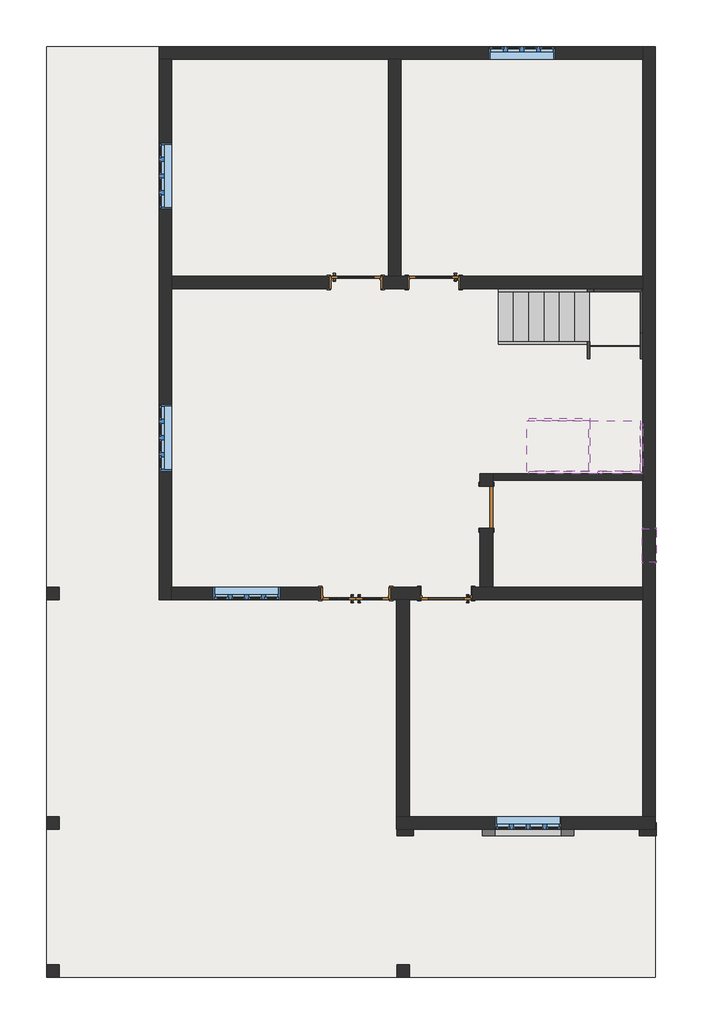
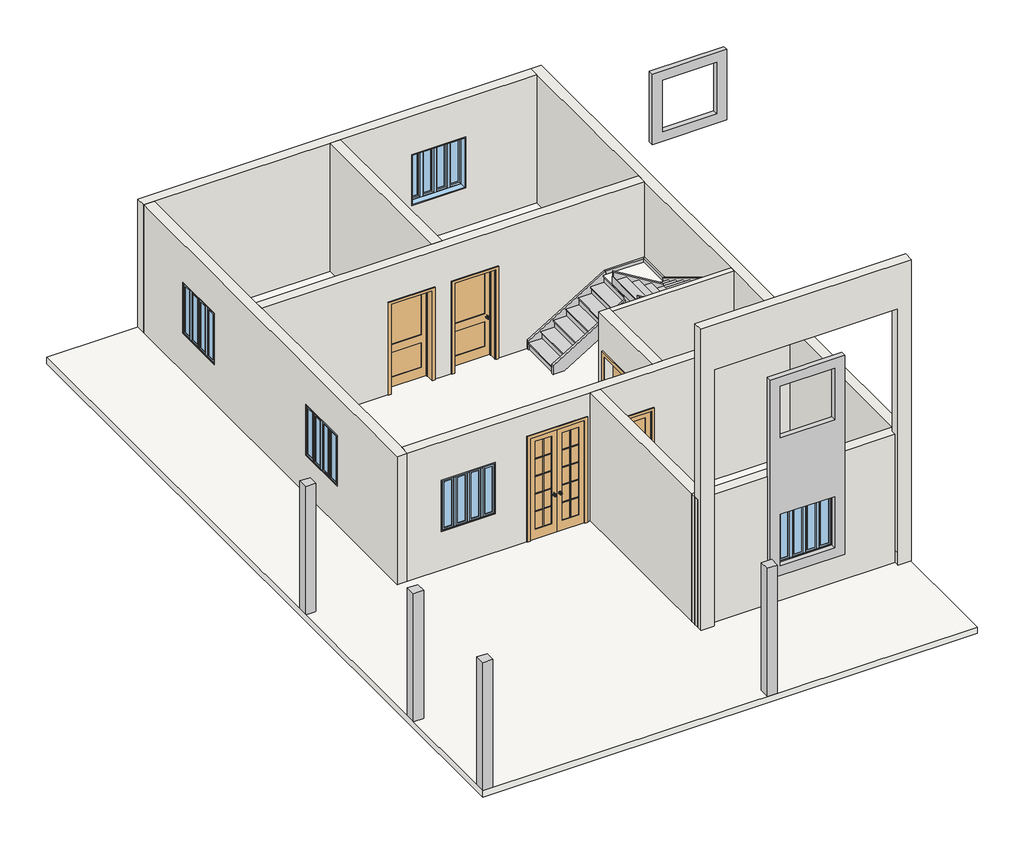
# One storey: 11 walls, 10 members, 6 columns, 6 windows, 5 doors, 3 slabs, 3 stair flights, 1 proxy.
"""IFC4 building model written with IfcOpenShell, lengths in millimetres."""

from ifc_helpers import new_model, si_unit, frame, origin, origin_with_axes, place, context, project, spatial, polyline, outline, extrude, faceted_brep, transform, mapped, element, save
from components import generic_models_1_generic_models_1_5e281b0c, door_interior_double_full_glass_wood_4_x_8_door_7870f6d1, door_interior_single_2_panel_wood_3_x_7_door_08fe406f, door_interior_single_2_panel_wood_3_x_7_door_700963f9, door_e31f6e4d, non_monolithic_landing_245f9fea, non_monolithic_landing_4f0ba0af, stair_flight_dd3871da, stair_flight_788f3b80, stair_flight_82b2d532, window_casement_multi_sash_horizontal_4_x_4_8de01852, window_6da96920

model = new_model("IFC4")

# Units and contexts
model_context = context("Model", 3, world=origin())
ifc_project = project(units=[si_unit("LENGTHUNIT", "METRE", prefix="MILLI")], contexts=[model_context])

# Site, building, storey
site = spatial("IfcSite", under=ifc_project)
building = spatial("IfcBuilding", under=site)
storey = spatial("IfcBuildingStorey", under=building, Elevation=0.0)

# Proxy
placement = place(None, origin())
generic_models_1_generic_models_1_shape = generic_models_1_generic_models_1_5e281b0c(model_context)
element("IfcBuildingElementProxy", 1, Name="Generic Models 1 : Generic Models 1", ObjectType="Generic Models 1 : Generic Models 1", at=placement, inside=storey, context=model_context, shape_type="MappedRepresentation", body=[
    mapped(generic_models_1_generic_models_1_shape, transform((0.0, 0.0, 0.0), x_axis=(1.0, 0.0, 0.0), y_axis=(0.0, 1.0, 0.0), z_axis=(0.0, 0.0, 1.0))),
])

# Columns
element("IfcColumn", 2, ObjectType="Rectangular Column : 9\" X 9\" COLUMN", at=placement, inside=storey, context=model_context, shape_type="SweptSolid", body=[
    extrude(outline(polyline([(-4334.4608498, -5108.7884134), (-4105.8608498, -5108.7884134), (-4105.8608498, -5222.3884134), (-4334.4608498, -5222.3884134), (-4334.4608498, -5108.7884134)])), origin_with_axes(), (0.0, 0.0, 1.0), 3048.0),
])
element("IfcColumn", 3, ObjectType="Rectangular Column : 9\" X 9\" COLUMN", at=placement, inside=storey, context=model_context, shape_type="SweptSolid", body=[
    extrude(outline(polyline([(-4105.8608498, -916.3884134), (-4105.8608498, -1144.9884134), (-4334.4608498, -1144.9884134), (-4334.4608498, -916.3884134), (-4105.8608498, -916.3884134)])), origin_with_axes(), (0.0, 0.0, 1.0), 3048.0),
])
element("IfcColumn", 4, ObjectType="Rectangular Column : 9\" X 9\" COLUMN", at=placement, inside=storey, context=model_context, shape_type="SweptSolid", body=[
    extrude(outline(polyline([(-10504.5608498, -916.3884134), (-10504.5608498, -1144.9884134), (-10733.1608498, -1144.9884134), (-10733.1608498, -916.3884134), (-10504.5608498, -916.3884134)])), origin_with_axes(), (0.0, 0.0, 1.0), 3048.0),
])
element("IfcColumn", 5, ObjectType="Rectangular Column : 9\" X 9\" COLUMN", at=placement, inside=storey, context=model_context, shape_type="SweptSolid", body=[
    extrude(outline(polyline([(-10504.5608498, -5108.7884134), (-10504.5608498, -5337.3884134), (-10733.1608498, -5337.3884134), (-10733.1608498, -5108.7884134), (-10504.5608498, -5108.7884134)])), origin_with_axes(), (0.0, 0.0, 1.0), 3048.0),
])
element("IfcColumn", 6, ObjectType="Rectangular Column : 9\" X 9\" COLUMN", at=placement, inside=storey, context=model_context, shape_type="SweptSolid", body=[
    extrude(outline(polyline([(-4105.8608498, -7814.5884134), (-4105.8608498, -8043.1884134), (-4334.4608498, -8043.1884134), (-4334.4608498, -7814.5884134), (-4105.8608498, -7814.5884134)])), origin_with_axes(), (0.0, 0.0, 1.0), 3048.0),
])
element("IfcColumn", 7, ObjectType="Rectangular Column : 9\" X 9\" COLUMN", at=placement, inside=storey, context=model_context, shape_type="SweptSolid", body=[
    extrude(outline(polyline([(-10504.5608498, -7814.5884134), (-10504.5608498, -8043.1884134), (-10733.1608498, -8043.1884134), (-10733.1608498, -7814.5884134), (-10504.5608498, -7814.5884134)])), origin_with_axes(), (0.0, 0.0, 1.0), 3048.0),
])

# Doors
door_interior_double_full_glass_wood_4_x_8_door_shape = door_interior_double_full_glass_wood_4_x_8_door_7870f6d1(model_context)
element("IfcDoor", 8, ObjectType="Door-Interior-Double-Full Glass-Wood : 4' X 8' DOOR", at=placement, inside=storey, context=model_context, shape_type="MappedRepresentation", body=[
    mapped(door_interior_double_full_glass_wood_4_x_8_door_shape, transform((-5084.4608498, -1033.8634134, 0.0), x_axis=(-1.0, 0.0, 0.0), y_axis=(0.0, -1.0, 0.0), z_axis=(0.0, 0.0, 1.0))),
])
door_interior_single_2_panel_wood_3_x_7_door_shape = door_interior_single_2_panel_wood_3_x_7_door_08fe406f(model_context)
element("IfcDoor", 9, ObjectType="Door-Interior-Single-2_Panel-Wood : 3' x 7' door", at=placement, inside=storey, context=model_context, shape_type="MappedRepresentation", body=[
    mapped(door_interior_single_2_panel_wood_3_x_7_door_shape, transform((-3430.6608498, -1033.8634134, 0.0), x_axis=(-1.0, 0.0, 0.0), y_axis=(0.0, -1.0, 0.0), z_axis=(0.0, 0.0, 1.0))),
])
element("IfcDoor", 10, ObjectType="Door-Interior-Single-2_Panel-Wood : 3' x 7' door", at=placement, inside=storey, context=model_context, shape_type="MappedRepresentation", body=[
    mapped(door_interior_single_2_panel_wood_3_x_7_door_shape, transform((-5081.6608498, 4648.6865866, 0.0), x_axis=(1.0, 0.0, 0.0), y_axis=(0.0, 1.0, 0.0), z_axis=(0.0, 0.0, 1.0))),
])
door_interior_single_2_panel_wood_3_x_7_door_2_shape = door_interior_single_2_panel_wood_3_x_7_door_700963f9(model_context)
element("IfcDoor", 11, ObjectType="Door-Interior-Single-2_Panel-Wood : 3' x 7' door", at=placement, inside=storey, context=model_context, shape_type="MappedRepresentation", body=[
    mapped(door_interior_single_2_panel_wood_3_x_7_door_2_shape, transform((-3657.8608498, 4648.6865866, 0.0), x_axis=(-1.0, 0.0, 0.0), y_axis=(0.0, -1.0, 0.0), z_axis=(0.0, 0.0, 1.0))),
])
door_shape = door_e31f6e4d(model_context)
element("IfcDoor", 12, ObjectType="Single-Flush : 2'6\" x 7'", at=placement, inside=storey, context=model_context, shape_type="MappedRepresentation", body=[
    mapped(door_shape, transform((-2696.1608498, 542.7115866, 0.0), x_axis=(0.0, 1.0, 0.0), y_axis=(-1.0, 0.0, 0.0), z_axis=(0.0, 0.0, 1.0))),
])

# Members
element("IfcMember", 13, ObjectType="Stringer - 2\" Width", at=placement, inside=storey, context=model_context, shape_type="SweptSolid", body=[
    extrude(outline(polyline([(212.114512, -2479.5608498), (0.0, -2479.5608498), (0.0, -2241.475338), (956.7333333, -662.865338), (1261.5333333, -748.0197945), (212.114512, -2479.5608498)])), frame((0.0, 4479.7115866, 0.0), z_axis=(0.0, 1.0, 0.0), x_axis=(0.0, 0.0, 1.0)), (0.0, 0.0, 1.0), 50.8),
])
element("IfcMember", 14, ObjectType="Stringer - 2\" Width", at=placement, inside=storey, context=model_context, shape_type="SweptSolid", body=[
    extrude(outline(polyline([(212.114512, -2479.5608498), (0.0, -2479.5608498), (0.0, -2241.475338), (840.9178717, -853.9608498), (1197.3266332, -853.9608498), (212.114512, -2479.5608498)])), frame((0.0, 3514.5115866, 0.0), z_axis=(0.0, 1.0, 0.0), x_axis=(0.0, 0.0, 1.0)), (0.0, 0.0, 1.0), 50.8),
])
element("IfcMember", 15, ObjectType="Stringer - 2\" Width", at=placement, inside=storey, context=model_context, shape_type="SweptSolid", body=[
    extrude(outline(polyline([(3738.7705314, 1261.5333333), (3653.6160748, 956.7333333), (1977.2160748, 1972.7333333), (2062.3705314, 2277.5333333), (3738.7705314, 1261.5333333)])), frame((111.2391502, 0.0, 0.0), z_axis=(1.0, 0.0, 0.0), x_axis=(0.0, 1.0, 0.0)), (0.0, 0.0, 1.0), 50.8),
])
element("IfcMember", 16, ObjectType="Stringer - 2\" Width", at=placement, inside=storey, context=model_context, shape_type="Brep", body=[
    faceted_brep([(-803.1608498, 3565.3115866, 1366.6599665), (-853.9608498, 3565.3115866, 1366.6599665), (-853.9608498, 2168.3115866, 2213.3266332), (-803.1608498, 2168.3115866, 2213.3266332), (-803.1608498, 3565.3115866, 1010.251205), (-803.1608498, 2168.3115866, 2057.0390838), (-803.1608498, 2168.3115866, 1856.9178717), (-853.9608498, 3565.3115866, 1010.251205), (-853.9608498, 2168.3115866, 1856.9178717)], [[[0, 1, 2, 3]], [[4, 0, 3, 5, 6]], [[7, 4, 6, 8]], [[1, 7, 8, 2]], [[1, 0, 4, 7]], [[2, 8, 6, 5, 3]]]),
])
element("IfcMember", 17, ObjectType="Stringer - 2\" Width", at=placement, inside=storey, context=model_context, shape_type="Brep", body=[
    faceted_brep([(111.2391502, 3738.7705314, 1261.5333333), (162.0391502, 3738.7705314, 1261.5333333), (162.0391502, 4530.5115866, 1261.5333333), (111.2391502, 4479.7115866, 1261.5333333), (111.2391502, 3653.6160748, 956.7333333), (111.2391502, 4479.7115866, 956.7333333), (162.0391502, 3653.6160748, 956.7333333), (162.0391502, 4530.5115866, 956.7333333)], [[[0, 1, 2, 3]], [[4, 0, 3, 5]], [[6, 4, 5, 7]], [[1, 6, 7, 2]], [[1, 0, 4, 6]], [[2, 7, 5, 3]]]),
])
element("IfcMember", 18, ObjectType="Stringer - 2\" Width", at=placement, inside=storey, context=model_context, shape_type="Brep", body=[
    faceted_brep([(111.2391502, 4479.7115866, 1261.5333333), (162.0391502, 4530.5115866, 1261.5333333), (-748.0197945, 4530.5115866, 1261.5333333), (-748.0197945, 4479.7115866, 1261.5333333), (111.2391502, 4479.7115866, 956.7333333), (-662.865338, 4479.7115866, 956.7333333), (162.0391502, 4530.5115866, 956.7333333), (-662.865338, 4530.5115866, 956.7333333)], [[[0, 1, 2, 3]], [[4, 0, 3, 5]], [[6, 4, 5, 7]], [[1, 6, 7, 2]], [[1, 0, 4, 6]], [[2, 7, 5, 3]]]),
])
element("IfcMember", 19, ObjectType="Stringer - 2\" Width", at=placement, inside=storey, context=model_context, shape_type="SweptSolid", body=[
    extrude(outline(polyline([(1972.7333333, -664.0563615), (2277.5333333, -578.901905), (3090.7811786, -1920.7608498), (2734.3724171, -1920.7608498), (1972.7333333, -664.0563615)])), frame((0.0, 1152.3115866, 0.0), z_axis=(0.0, 1.0, 0.0), x_axis=(0.0, 0.0, 1.0)), (0.0, 0.0, 1.0), 50.8),
])
element("IfcMember", 20, ObjectType="Stringer - 2\" Width", at=placement, inside=storey, context=model_context, shape_type="Brep", body=[
    faceted_brep([(-1920.7608498, 2168.3115866, 3090.7811786), (-1920.7608498, 2168.3115866, 2734.3724171), (-1920.7608498, 2117.5115866, 2734.3724171), (-1920.7608498, 2117.5115866, 3090.7811786), (-803.1608498, 2117.5115866, 2413.4478453), (-803.1608498, 2168.3115866, 2413.4478453), (-803.1608498, 2117.5115866, 2057.0390838), (-803.1608498, 2168.3115866, 2057.0390838), (-803.1608498, 2168.3115866, 2213.3266332)], [[[0, 1, 2, 3]], [[4, 5, 0, 3]], [[6, 4, 3, 2]], [[7, 6, 2, 1]], [[5, 8, 7, 1, 0]], [[5, 4, 6, 7, 8]]]),
])
element("IfcMember", 21, ObjectType="Stringer - 2\" Width", at=placement, inside=storey, context=model_context, shape_type="Brep", body=[
    faceted_brep([(-578.901905, 1203.1115866, 2277.5333333), (-578.901905, 1152.3115866, 2277.5333333), (162.0391502, 1152.3115866, 2277.5333333), (111.2391502, 1203.1115866, 2277.5333333), (-664.0563615, 1203.1115866, 1972.7333333), (111.2391502, 1203.1115866, 1972.7333333), (-664.0563615, 1152.3115866, 1972.7333333), (162.0391502, 1152.3115866, 1972.7333333)], [[[0, 1, 2, 3]], [[4, 0, 3, 5]], [[6, 4, 5, 7]], [[1, 6, 7, 2]], [[1, 0, 4, 6]], [[2, 7, 5, 3]]]),
])
element("IfcMember", 22, ObjectType="Stringer - 2\" Width", at=placement, inside=storey, context=model_context, shape_type="Brep", body=[
    faceted_brep([(111.2391502, 1203.1115866, 2277.5333333), (162.0391502, 1152.3115866, 2277.5333333), (162.0391502, 2062.3705314, 2277.5333333), (111.2391502, 2062.3705314, 2277.5333333), (111.2391502, 1203.1115866, 1972.7333333), (111.2391502, 1977.2160748, 1972.7333333), (162.0391502, 1152.3115866, 1972.7333333), (162.0391502, 1977.2160748, 1972.7333333)], [[[0, 1, 2, 3]], [[4, 0, 3, 5]], [[6, 4, 5, 7]], [[1, 6, 7, 2]], [[1, 0, 4, 6]], [[2, 7, 5, 3]]]),
])

# Slabs
element("IfcSlab", 23, ObjectType="6\" FLOOR", at=placement, inside=storey, context=model_context, shape_type="SweptSolid", body=[
    extrude(outline(polyline([(-10733.1608498, 8952.9115866), (392.0391502, 8952.9115866), (392.0391502, -8043.1884134), (-10733.1608498, -8043.1884134), (-10733.1608498, 8952.9115866)])), frame((0.0, 0.0, -152.4), z_axis=(0.0, 0.0, 1.0), x_axis=(1.0, 0.0, 0.0)), (0.0, 0.0, 1.0), 152.4),
])
non_monolithic_landing_shape = non_monolithic_landing_245f9fea(model_context)
element("IfcSlab", 24, ObjectType="Non-Monolithic Landing", at=placement, inside=storey, context=model_context, shape_type="MappedRepresentation", body=[
    mapped(non_monolithic_landing_shape, transform((0.0, 0.0, 0.0), x_axis=(1.0, 0.0, 0.0), y_axis=(0.0, 1.0, 0.0), z_axis=(0.0, 0.0, 1.0))),
])
non_monolithic_landing_2_shape = non_monolithic_landing_4f0ba0af(model_context)
element("IfcSlab", 25, ObjectType="Non-Monolithic Landing", at=placement, inside=storey, context=model_context, shape_type="MappedRepresentation", body=[
    mapped(non_monolithic_landing_2_shape, transform((0.0, 0.0, 0.0), x_axis=(1.0, 0.0, 0.0), y_axis=(0.0, 1.0, 0.0), z_axis=(0.0, 0.0, 1.0))),
])

# Stair flights
stair_flight_shape = stair_flight_dd3871da(model_context)
element("IfcStairFlight", 26, ObjectType="2\" Tread 1\" Nosing 1/4\" Riser", at=placement, inside=storey, context=model_context, shape_type="MappedRepresentation", body=[
    mapped(stair_flight_shape, transform((0.0, 0.0, 0.0), x_axis=(1.0, 0.0, 0.0), y_axis=(0.0, 1.0, 0.0), z_axis=(0.0, 0.0, 1.0))),
])
stair_flight_2_shape = stair_flight_788f3b80(model_context)
element("IfcStairFlight", 27, ObjectType="2\" Tread 1\" Nosing 1/4\" Riser", at=placement, inside=storey, context=model_context, shape_type="MappedRepresentation", body=[
    mapped(stair_flight_2_shape, transform((0.0, 0.0, 0.0), x_axis=(1.0, 0.0, 0.0), y_axis=(0.0, 1.0, 0.0), z_axis=(0.0, 0.0, 1.0))),
])
stair_flight_3_shape = stair_flight_82b2d532(model_context)
element("IfcStairFlight", 28, ObjectType="2\" Tread 1\" Nosing 1/4\" Riser", at=placement, inside=storey, context=model_context, shape_type="MappedRepresentation", body=[
    mapped(stair_flight_3_shape, transform((0.0, 0.0, 0.0), x_axis=(1.0, 0.0, 0.0), y_axis=(0.0, 1.0, 0.0), z_axis=(0.0, 0.0, 1.0))),
])

# Walls
element("IfcWall", 29, ObjectType="4.5\" wall", at=placement, inside=storey, context=model_context, shape_type="SweptSolid", body=[
    extrude(outline(polyline([(162.0391502, 1038.0115866), (-2581.1608498, 1038.0115866), (-2581.1608498, 1152.3115866), (162.0391502, 1152.3115866), (162.0391502, 1038.0115866)])), origin_with_axes(), (0.0, 0.0, 1.0), 3048.0),
])
element("IfcWall", 30, ObjectType="9\" wall", at=placement, inside=storey, context=model_context, shape_type="Brep", body=[
    faceted_brep([(-4335.1608498, -5338.0884134, 0.0), (392.0391502, -5338.0884134, 0.0), (392.0391502, -5338.0884134, 3048.0), (-4335.1608498, -5338.0884134, 3048.0), (-2542.3608498, -5338.0884134, 2133.6), (-1323.1608498, -5338.0884134, 2133.6), (-1323.1608498, -5338.0884134, 914.4), (-2542.3608498, -5338.0884134, 914.4), (-4335.1608498, -5108.0884134, 0.0), (-4335.1608498, -5108.0884134, 3048.0), (-4105.1608498, -5108.0884134, 3048.0), (162.0391502, -5108.0884134, 3048.0), (392.0391502, -5108.0884134, 3048.0), (392.0391502, -5108.0884134, 0.0), (162.0391502, -5108.0884134, 0.0), (-4105.1608498, -5108.0884134, 0.0), (-2542.3608498, -5108.0884134, 2133.6), (-2542.3608498, -5108.0884134, 914.4), (-1323.1608498, -5108.0884134, 914.4), (-1323.1608498, -5108.0884134, 2133.6)], [[[0, 1, 2, 3], [4, 5, 6, 7]], [[8, 9, 10, 11, 12, 13, 14, 15], [16, 17, 18, 19]], [[1, 0, 8, 15, 14, 13]], [[3, 2, 12, 11, 10, 9]], [[17, 16, 4, 7]], [[18, 17, 7, 6]], [[19, 18, 6, 5]], [[16, 19, 5, 4]], [[2, 1, 13, 12]], [[0, 3, 9, 8]]]),
])
element("IfcWall", 31, ObjectType="9\" wall", at=placement, inside=storey, context=model_context, shape_type="Brep", body=[
    faceted_brep([(392.0391502, -5108.0884134, 0.0), (392.0391502, 8952.9115866, 0.0), (392.0391502, 8952.9115866, 3048.0), (392.0391502, 1155.1115866, 3048.0), (392.0391502, -5108.0884134, 3048.0), (392.0391502, 151.1115866, 2133.6), (392.0391502, 151.1115866, 1524.0), (392.0391502, -458.4884134, 1524.0), (392.0391502, -458.4884134, 2133.6), (162.0391502, -5108.0884134, 0.0), (162.0391502, -5108.0884134, 3048.0), (162.0391502, -1145.6884134, 3048.0), (162.0391502, -915.6884134, 3048.0), (162.0391502, 1038.0115866, 3048.0), (162.0391502, 1152.3115866, 3048.0), (162.0391502, 1155.1115866, 3048.0), (162.0391502, 4530.5115866, 3048.0), (162.0391502, 4760.5115866, 3048.0), (162.0391502, 8722.9115866, 3048.0), (162.0391502, 8952.9115866, 3048.0), (162.0391502, 8952.9115866, 0.0), (162.0391502, 8722.9115866, 0.0), (162.0391502, 4760.5115866, 0.0), (162.0391502, 4530.5115866, 0.0), (162.0391502, 1152.3115866, 0.0), (162.0391502, 1038.0115866, 0.0), (162.0391502, -915.6884134, 0.0), (162.0391502, -1145.6884134, 0.0), (162.0391502, 151.1115866, 2133.6), (162.0391502, -458.4884134, 2133.6), (162.0391502, -458.4884134, 1524.0), (162.0391502, 151.1115866, 1524.0)], [[[0, 1, 2, 3, 4], [5, 6, 7, 8]], [[9, 10, 11, 12, 13, 14, 15, 16, 17, 18, 19, 20, 21, 22, 23, 24, 25, 26, 27], [28, 29, 30, 31]], [[1, 0, 9, 27, 26, 25, 24, 23, 22, 21, 20]], [[4, 3, 2, 19, 18, 17, 16, 15, 14, 13, 12, 11, 10]], [[2, 1, 20, 19]], [[6, 5, 28, 31]], [[7, 6, 31, 30]], [[8, 7, 30, 29]], [[5, 8, 29, 28]], [[0, 4, 10, 9]]]),
])
element("IfcWall", 32, ObjectType="9\" wall", at=placement, inside=storey, context=model_context, shape_type="Brep", body=[
    faceted_brep([(162.0391502, 8952.9115866, 0.0), (-8677.1608498, 8952.9115866, 0.0), (-8677.1608498, 8952.9115866, 3048.0), (162.0391502, 8952.9115866, 3048.0), (-1436.7608498, 8952.9115866, 2133.6), (-2655.9608498, 8952.9115866, 2133.6), (-2655.9608498, 8952.9115866, 914.4), (-1436.7608498, 8952.9115866, 914.4), (162.0391502, 8722.9115866, 0.0), (162.0391502, 8722.9115866, 3048.0), (-4254.7608498, 8722.9115866, 3048.0), (-4484.7608498, 8722.9115866, 3048.0), (-8447.1608498, 8722.9115866, 3048.0), (-8677.1608498, 8722.9115866, 3048.0), (-8677.1608498, 8722.9115866, 0.0), (-8447.1608498, 8722.9115866, 0.0), (-4484.7608498, 8722.9115866, 0.0), (-4254.7608498, 8722.9115866, 0.0), (-1436.7608498, 8722.9115866, 2133.6), (-1436.7608498, 8722.9115866, 914.4), (-2655.9608498, 8722.9115866, 914.4), (-2655.9608498, 8722.9115866, 2133.6)], [[[0, 1, 2, 3], [4, 5, 6, 7]], [[8, 9, 10, 11, 12, 13, 14, 15, 16, 17], [18, 19, 20, 21]], [[1, 0, 8, 17, 16, 15, 14]], [[3, 2, 13, 12, 11, 10, 9]], [[0, 3, 9, 8]], [[2, 1, 14, 13]], [[19, 18, 4, 7]], [[20, 19, 7, 6]], [[21, 20, 6, 5]], [[18, 21, 5, 4]]]),
])
element("IfcWall", 33, ObjectType="9\" wall", at=placement, inside=storey, context=model_context, shape_type="Brep", body=[
    faceted_brep([(-8677.1608498, 8722.9115866, 0.0), (-8677.1608498, -1145.6884134, 0.0), (-8677.1608498, -1145.6884134, 3048.0), (-8677.1608498, 8722.9115866, 3048.0), (-8677.1608498, 7198.9115866, 2133.6), (-8677.1608498, 5979.7115866, 2133.6), (-8677.1608498, 5979.7115866, 914.4), (-8677.1608498, 7198.9115866, 914.4), (-8677.1608498, 2417.0115866, 2133.6), (-8677.1608498, 1197.8115866, 2133.6), (-8677.1608498, 1197.8115866, 914.4), (-8677.1608498, 2417.0115866, 914.4), (-8447.1608498, 8722.9115866, 0.0), (-8447.1608498, 8722.9115866, 3048.0), (-8447.1608498, 4760.5115866, 3048.0), (-8447.1608498, 4530.5115866, 3048.0), (-8447.1608498, -915.6884134, 3048.0), (-8447.1608498, -1145.6884134, 3048.0), (-8447.1608498, -1145.6884134, 0.0), (-8447.1608498, -915.6884134, 0.0), (-8447.1608498, 4530.5115866, 0.0), (-8447.1608498, 4760.5115866, 0.0), (-8447.1608498, 7198.9115866, 2133.6), (-8447.1608498, 7198.9115866, 914.4), (-8447.1608498, 5979.7115866, 914.4), (-8447.1608498, 5979.7115866, 2133.6), (-8447.1608498, 2417.0115866, 2133.6), (-8447.1608498, 2417.0115866, 914.4), (-8447.1608498, 1197.8115866, 914.4), (-8447.1608498, 1197.8115866, 2133.6)], [[[0, 1, 2, 3], [4, 5, 6, 7], [8, 9, 10, 11]], [[12, 13, 14, 15, 16, 17, 18, 19, 20, 21], [22, 23, 24, 25], [26, 27, 28, 29]], [[1, 0, 12, 21, 20, 19, 18]], [[3, 2, 17, 16, 15, 14, 13]], [[0, 3, 13, 12]], [[2, 1, 18, 17]], [[23, 22, 4, 7]], [[24, 23, 7, 6]], [[25, 24, 6, 5]], [[22, 25, 5, 4]], [[27, 26, 8, 11]], [[28, 27, 11, 10]], [[29, 28, 10, 9]], [[26, 29, 9, 8]]]),
])
element("IfcWall", 34, ObjectType="9\" wall", at=placement, inside=storey, context=model_context, shape_type="Brep", body=[
    faceted_brep([(-8447.1608498, 4760.5115866, 3048.0), (-4484.7608498, 4760.5115866, 3048.0), (-4254.7608498, 4760.5115866, 3048.0), (162.0391502, 4760.5115866, 3048.0), (162.0391502, 4760.5115866, 0.0), (-3175.2608498, 4760.5115866, 0.0), (-3175.2608498, 4760.5115866, 2159.0), (-4140.4608498, 4760.5115866, 2159.0), (-4140.4608498, 4760.5115866, 0.0), (-4254.7608498, 4760.5115866, 0.0), (-4484.7608498, 4760.5115866, 0.0), (-4599.0608498, 4760.5115866, 0.0), (-4599.0608498, 4760.5115866, 2159.0), (-5564.2608498, 4760.5115866, 2159.0), (-5564.2608498, 4760.5115866, 0.0), (-8447.1608498, 4760.5115866, 0.0), (162.0391502, 4530.5115866, 3048.0), (-8447.1608498, 4530.5115866, 3048.0), (-8447.1608498, 4530.5115866, 0.0), (-5564.2608498, 4530.5115866, 0.0), (-5564.2608498, 4530.5115866, 2159.0), (-4599.0608498, 4530.5115866, 2159.0), (-4599.0608498, 4530.5115866, 0.0), (-4140.4608498, 4530.5115866, 0.0), (-4140.4608498, 4530.5115866, 2159.0), (-3175.2608498, 4530.5115866, 2159.0), (-3175.2608498, 4530.5115866, 0.0), (162.0391502, 4530.5115866, 0.0)], [[[0, 1, 2, 3, 4, 5, 6, 7, 8, 9, 10, 11, 12, 13, 14, 15]], [[16, 17, 18, 19, 20, 21, 22, 23, 24, 25, 26, 27]], [[4, 27, 26, 5]], [[18, 15, 14, 19]], [[22, 11, 10, 9, 8, 23]], [[3, 2, 1, 0, 17, 16]], [[4, 3, 16, 27]], [[0, 15, 18, 17]], [[21, 12, 11, 22]], [[12, 21, 20, 13]], [[13, 20, 19, 14]], [[7, 24, 23, 8]], [[24, 7, 6, 25]], [[25, 6, 5, 26]]]),
])
element("IfcWall", 35, ObjectType="9\" wall", at=placement, inside=storey, context=model_context, shape_type="SweptSolid", body=[
    extrude(outline(polyline([(-4484.7608498, 4760.5115866), (-4484.7608498, 8722.9115866), (-4254.7608498, 8722.9115866), (-4254.7608498, 4760.5115866), (-4484.7608498, 4760.5115866)])), origin_with_axes(), (0.0, 0.0, 1.0), 3048.0),
])
element("IfcWall", 36, ObjectType="9\" wall", at=placement, inside=storey, context=model_context, shape_type="Brep", body=[
    faceted_brep([(162.0391502, -1145.6884134, 3048.0), (-4105.1608498, -1145.6884134, 3048.0), (-4335.1608498, -1145.6884134, 3048.0), (-8447.1608498, -1145.6884134, 3048.0), (-8447.1608498, -1145.6884134, 0.0), (-5719.4608498, -1145.6884134, 0.0), (-5719.4608498, -1145.6884134, 2463.8), (-4449.4608498, -1145.6884134, 2463.8), (-4449.4608498, -1145.6884134, 0.0), (-4335.1608498, -1145.6884134, 0.0), (-4105.1608498, -1145.6884134, 0.0), (-3913.2608498, -1145.6884134, 0.0), (-3913.2608498, -1145.6884134, 2159.0), (-2948.0608498, -1145.6884134, 2159.0), (-2948.0608498, -1145.6884134, 0.0), (162.0391502, -1145.6884134, 0.0), (-7685.1608498, -1145.6884134, 2133.6), (-6465.9608498, -1145.6884134, 2133.6), (-6465.9608498, -1145.6884134, 914.4), (-7685.1608498, -1145.6884134, 914.4), (-8447.1608498, -915.6884134, 3048.0), (-2811.1608498, -915.6884134, 3048.0), (-2581.1608498, -915.6884134, 3048.0), (162.0391502, -915.6884134, 3048.0), (162.0391502, -915.6884134, 0.0), (-2581.1608498, -915.6884134, 0.0), (-2811.1608498, -915.6884134, 0.0), (-2948.0608498, -915.6884134, 0.0), (-2948.0608498, -915.6884134, 2159.0), (-3913.2608498, -915.6884134, 2159.0), (-3913.2608498, -915.6884134, 0.0), (-4449.4608498, -915.6884134, 0.0), (-4449.4608498, -915.6884134, 2463.8), (-5719.4608498, -915.6884134, 2463.8), (-5719.4608498, -915.6884134, 0.0), (-8447.1608498, -915.6884134, 0.0), (-7685.1608498, -915.6884134, 2133.6), (-7685.1608498, -915.6884134, 914.4), (-6465.9608498, -915.6884134, 914.4), (-6465.9608498, -915.6884134, 2133.6)], [[[0, 1, 2, 3, 4, 5, 6, 7, 8, 9, 10, 11, 12, 13, 14, 15], [16, 17, 18, 19]], [[20, 21, 22, 23, 24, 25, 26, 27, 28, 29, 30, 31, 32, 33, 34, 35], [36, 37, 38, 39]], [[24, 15, 14, 27, 26, 25]], [[4, 35, 34, 5]], [[30, 11, 10, 9, 8, 31]], [[3, 2, 1, 0, 23, 22, 21, 20]], [[0, 15, 24, 23]], [[4, 3, 20, 35]], [[29, 12, 11, 30]], [[12, 29, 28, 13]], [[13, 28, 27, 14]], [[37, 36, 16, 19]], [[38, 37, 19, 18]], [[39, 38, 18, 17]], [[36, 39, 17, 16]], [[33, 6, 5, 34]], [[6, 33, 32, 7]], [[7, 32, 31, 8]]]),
])
element("IfcWall", 37, ObjectType="9\" wall", at=placement, inside=storey, context=model_context, shape_type="SweptSolid", body=[
    extrude(outline(polyline([(-4105.1608498, -1145.6884134), (-4105.1608498, -5108.0884134), (-4335.1608498, -5108.0884134), (-4335.1608498, -1145.6884134), (-4105.1608498, -1145.6884134)])), origin_with_axes(), (0.0, 0.0, 1.0), 3048.0),
])
element("IfcWall", 38, ObjectType="9\" wall", at=placement, inside=storey, context=model_context, shape_type="Brep", body=[
    faceted_brep([(-2811.1608498, 1152.3115866, 0.0), (-2811.1608498, 923.7115866, 0.0), (-2811.1608498, 923.7115866, 2133.6), (-2811.1608498, 161.7115866, 2133.6), (-2811.1608498, 161.7115866, 0.0), (-2811.1608498, -915.6884134, 0.0), (-2811.1608498, -915.6884134, 3048.0), (-2811.1608498, 1152.3115866, 3048.0), (-2581.1608498, 923.7115866, 2133.6), (-2581.1608498, 923.7115866, 0.0), (-2581.1608498, 1038.0115866, 0.0), (-2581.1608498, 1152.3115866, 0.0), (-2581.1608498, 1152.3115866, 3048.0), (-2581.1608498, 1038.0115866, 3048.0), (-2581.1608498, -915.6884134, 3048.0), (-2581.1608498, -915.6884134, 0.0), (-2581.1608498, 161.7115866, 0.0), (-2581.1608498, 161.7115866, 2133.6)], [[[0, 1, 2, 3, 4, 5, 6, 7]], [[8, 9, 10, 11, 12, 13, 14, 15, 16, 17]], [[16, 15, 5, 4]], [[11, 10, 9, 1, 0]], [[7, 6, 14, 13, 12]], [[6, 5, 15, 14]], [[0, 7, 12, 11]], [[2, 1, 9, 8]], [[3, 2, 8, 17]], [[4, 3, 17, 16]]]),
])
element("IfcWall", 39, ObjectType="9\" wall", at=placement, inside=storey, context=model_context, shape_type="Brep", body=[
    faceted_brep([(-4334.4608498, -5452.3884134, 0.0), (-4029.6608498, -5452.3884134, 0.0), (-4029.6608498, -5452.3884134, 304.8), (-4029.6608498, -5452.3884134, 6096.0), (99.2391502, -5452.3884134, 6096.0), (99.2391502, -5452.3884134, 304.8), (99.2391502, -5452.3884134, 0.0), (404.0391502, -5452.3884134, 0.0), (404.0391502, -5452.3884134, 7162.8), (-4334.4608498, -5452.3884134, 7162.8), (-4334.4608498, -5222.3884134, 0.0), (-4334.4608498, -5222.3884134, 3048.0), (-4334.4608498, -5222.3884134, 6096.0), (-4334.4608498, -5222.3884134, 7162.8), (404.0391502, -5222.3884134, 7162.8), (404.0391502, -5222.3884134, 0.0), (99.2391502, -5222.3884134, 0.0), (99.2391502, -5222.3884134, 304.8), (99.2391502, -5222.3884134, 6096.0), (-4029.6608498, -5222.3884134, 6096.0), (-4029.6608498, -5222.3884134, 304.8), (-4029.6608498, -5222.3884134, 0.0), (-4105.8608498, -5222.3884134, 0.0)], [[[0, 1, 2, 3, 4, 5, 6, 7, 8, 9]], [[10, 11, 12, 13, 14, 15, 16, 17, 18, 19, 20, 21, 22]], [[1, 0, 10, 22, 21]], [[8, 7, 15, 14]], [[9, 8, 14, 13]], [[0, 9, 13, 12, 11, 10]], [[2, 1, 21, 20]], [[3, 2, 20, 19]], [[4, 3, 19, 18]], [[5, 4, 18, 17]], [[6, 5, 17, 16]], [[7, 6, 16, 15]]]),
])

# Windows
window_casement_multi_sash_horizontal_4_x_4_shape = window_casement_multi_sash_horizontal_4_x_4_8de01852(model_context)
element("IfcWindow", 40, ObjectType="Window-Casement-Multi-Sash-Horizontal : 4' x 4'", at=placement, inside=storey, context=model_context, shape_type="MappedRepresentation", body=[
    mapped(window_casement_multi_sash_horizontal_4_x_4_shape, transform((-8562.1608498, 6589.3115866, 0.0), x_axis=(0.0, 1.0, 0.0), y_axis=(-1.0, 0.0, 0.0), z_axis=(0.0, 0.0, 1.0))),
])
element("IfcWindow", 41, ObjectType="Window-Casement-Multi-Sash-Horizontal : 4' x 4'", at=placement, inside=storey, context=model_context, shape_type="MappedRepresentation", body=[
    mapped(window_casement_multi_sash_horizontal_4_x_4_shape, transform((-2046.3608498, 8837.9115866, 0.0), x_axis=(1.0, 0.0, 0.0), y_axis=(0.0, 1.0, 0.0), z_axis=(0.0, 0.0, 1.0))),
])
element("IfcWindow", 42, ObjectType="Window-Casement-Multi-Sash-Horizontal : 4' x 4'", at=placement, inside=storey, context=model_context, shape_type="MappedRepresentation", body=[
    mapped(window_casement_multi_sash_horizontal_4_x_4_shape, transform((-8562.1608498, 1807.4115866, 0.0), x_axis=(0.0, 1.0, 0.0), y_axis=(-1.0, 0.0, 0.0), z_axis=(0.0, 0.0, 1.0))),
])
element("IfcWindow", 43, ObjectType="Window-Casement-Multi-Sash-Horizontal : 4' x 4'", at=placement, inside=storey, context=model_context, shape_type="MappedRepresentation", body=[
    mapped(window_casement_multi_sash_horizontal_4_x_4_shape, transform((-7075.5608498, -1030.6884134, 0.0), x_axis=(-1.0, 0.0, 0.0), y_axis=(0.0, -1.0, 0.0), z_axis=(0.0, 0.0, 1.0))),
])
element("IfcWindow", 44, ObjectType="Window-Casement-Multi-Sash-Horizontal : 4' x 4'", at=placement, inside=storey, context=model_context, shape_type="MappedRepresentation", body=[
    mapped(window_casement_multi_sash_horizontal_4_x_4_shape, transform((-1932.7608498, -5223.0884134, 0.0), x_axis=(-1.0, 0.0, 0.0), y_axis=(0.0, -1.0, 0.0), z_axis=(0.0, 0.0, 1.0))),
])
window_shape = window_6da96920(model_context)
element("IfcWindow", 45, ObjectType="Window-Louvers : 24\" x 24\"", at=placement, inside=storey, context=model_context, shape_type="MappedRepresentation", body=[
    mapped(window_shape, transform((283.3891502, -153.6884134, 609.6), x_axis=(0.0, -1.0, 0.0), y_axis=(1.0, 0.0, 0.0), z_axis=(0.0, 0.0, 1.0))),
])

save(model, "model.ifc")

# Revit data of these elements
# Grids (mm)
#   "1": line (-12064.335, 8837.912) -> (2480.906, 8837.912)
#   "2": line (-12064.335, 4645.512) -> (2480.906, 4645.512)
#   "4": line (-12064.335, -5223.088) -> (162.039, -5223.088)
#   "C": line (277.039, 10314.811) -> (277.039, -6476.174)
#   "D": line (-12064.335, 8837.912) -> (2480.906, 8837.912)
#   "E": line (-4369.761, 10314.811) -> (-4369.761, -6476.174)
#   "F": line (277.039, 10314.811) -> (277.039, -6476.174)
#   "B": line (-4369.761, 10314.811) -> (-4369.761, -6476.174)
#   "3": line (-12064.335, -1030.688) -> (162.039, -1030.688)
#   "A": line (-8562.161, 10314.811) -> (-8562.161, -6476.174)
# Type "Rectangular Column : 9\" X 9\" COLUMN"
#   Assembly Code = "B1010200"
#   Depth = 0' - 9"
#   Offset Base = 0' - 0"
#   Offset Top = 0' - 0"
#   Width = 0' - 9"
#   Material = none
# Type "Door-Interior-Double-Full Glass-Wood : 4' X 8' DOOR"
#   Type Mark = "12"
#   Assembly Code = "C1020300"
#   Analytic Construction = "French door, wood frame with single glass"
#   Top Rail = 0' - 4 11/16"
#   Thickness = 0' - 1 3/8"
#   Thermal Resistance (R) = 1.0696 (h·ft²·°F)/BTU
#   Swing Angle [instance default] = 90.00°
#   Stiles = 0' - 4 3/4"
#   Rough Width = 4' - 2"
#   Rough Height = 8' - 1"
#   Panel Width = 2' - 0"
#   Height = 8' - 0"
#   Width = 4' - 0"
#   Heat Transfer Coefficient (U) = 0.9350 BTU/(h·ft²·°F)
#   Bottom Rail = 0' - 9 1/8"
#   Show Grill [instance default] = yes
#   Trim Material = Cherry
#   Panel Material = Cherry
#   Frame Material = Cherry
#   Door Handle Material = Aluminum
#   Visual Light Transmittance = 0
#   Solar Heat Gain Coefficient = 0
#   Wall Closure = (empty or 0)
#   Function = (empty or 0)
# Type "Door-Interior-Single-2_Panel-Wood : 3' x 7' door"
#   Type Mark = "9"
#   Assembly Code = "C1020300"
#   Analytic Construction = "Wooden"
#   Top Rail = 0' - 4 11/16"
#   Thickness = 0' - 1 3/8"
#   Thermal Resistance (R) = 2.5876 (h·ft²·°F)/BTU
#   Swing Angle [instance default] = 90.00°
#   Stiles = 0' - 4 3/4"
#   Rough Width = 3' - 2"
#   Rough Height = 7' - 1"
#   Lock Rail = 0' - 7 1/2"
#   Height = 7' - 0"
#   Width = 3' - 0"
#   Heat Transfer Coefficient (U) = 0.3865 BTU/(h·ft²·°F)
#   Bottom Rail = 0' - 9 1/8"
#   Trim Material = Cherry
#   Panel Material = Cherry
#   Frame Material = Cherry
#   Door Handle Material = Aluminum
#   Visual Light Transmittance = 0
#   Solar Heat Gain Coefficient = 0
#   Wall Closure = (empty or 0)
#   Function = (empty or 0)
# Type "Single-Flush : 2'6\" x 7'"
#   Type Mark = "10"
#   Construction Type Id = "MDOOR"
#   Assembly Code = "C1020"
#   Analytic Construction = "Metal"
#   Thickness = 0' - 2"
#   Heat Transfer Coefficient (U) = 0.651978 BTU/(h·ft²·°F)
#   Height = 7' - 0"
#   Trim Projection Ext = 0' - 1"
#   Trim Projection Int = 0' - 1"
#   Trim Width = 0' - 3"
#   Width = 2' - 6"
#   Define Thermal Properties by = 1
#   Door Material = Door - Panel
#   Frame Material = Door - Frame
#   Visual Light Transmittance = 0
#   Solar Heat Gain Coefficient = 0
#   Function = (empty or 0)
#   Wall Closure = (empty or 0)
# Type "6\" FLOOR"
#   Assembly Code = "B1010"
#   Function = 0
#   Layers, outside or top first: 0' - 6" no material (function 1)
# Type "4.5\" wall"
#   Assembly Code = "B2010"
#   Layers, outside or top first: 0' - 4 1/2" no material (function 1)
# Type "9\" wall"
#   Assembly Code = "B2010"
#   Layers, outside or top first: 0' - 9 7/128" no material (function 1)
# Type "Window-Casement-Multi-Sash-Horizontal : 4' x 4'"
#   Type Mark = "W1"
#   Fire Rating = "0.5h"
#   Assembly Code = "B2020100"
#   Analytic Construction = "Double glazing - domestic"
#   Window Inset [instance default] = 0' - 0 5/8"
#   Wall Thickness [instance default] = 0' - 6"
#   Visual Light Transmittance = 0.81
#   Thermal Resistance (R) = 1.8146 (h·ft²·°F)/BTU
#   Solar Heat Gain Coefficient = 0.76
#   Rough Width = 4' - 0 1/2"
#   Rough Height = 4' - 0 1/2"
#   Open Window Width = 1' - 0"
#   Heat Transfer Coefficient (U) = 0.5511 BTU/(h·ft²·°F)
#   Height = 4' - 0"
#   Frame Gap 3 [instance default] = 0' - 1 83/128"
#   Frame Gap 2 [instance default] = 0' - 0 5/8"
#   Frame Gap 1 = 0' - 1 51/128"
#   Default Sill Height = 3' - 0"
#   Width = 4' - 0"
#   Frame Material = Metal - Aluminum
#   Glass Panel Material = Glass
#   Wall Closure = (empty or 0)
# Type "Window-Louvers : 24\" x 24\""
#   Type Mark = "V"
#   Construction Type Id = "GSP4R"
#   Assembly Code = "B20"
#   Analytic Construction = "1/8 in Pilkington single glazing"
#   Visual Light Transmittance = 0.9
#   Thermal Resistance (R) = 1.53941 (h·ft²·°F)/BTU
#   Solar Heat Gain Coefficient = 0.78
#   Max Height = 1' - 11.74264"
#   Height = 2' - 0"
#   Heat Transfer Coefficient (U) = 0.6496 BTU/(h·ft²·°F)
#   Blade Width [instance default] = 1' - 10 1/2"
#   Blade Vertical Thickness = 0' - 0.35355"
#   Blade Thickness = 0' - 0 1/4"
#   Blade Spacing = 0' - 1 1/2"
#   Blade Height = 0' - 1.85355"
#   Blade Depth = 0' - 3"
#   Blade Angle = 45.00°
#   Default Sill Height = 3' - 0"
#   Trim Projection_Exterior = 0' - 0 1/2"
#   Trim Projection_Interior = 0' - 0 1/2"
#   Trim Width_Exterior = 0' - 1 1/2"
#   Trim Width_Interior = 0' - 1 1/2"
#   Width = 2' - 0"
#   Max Blade Count = 12
#   Define Thermal Properties by = 1
#   Blade Count = 12
#   Frame Material = Birch
#   Louver Material = Birch
#   Trim Exterior Material = Birch
#   Trim Interior Material = Birch
#   Wall Closure = (empty or 0)
# Element 1 (IfcBuildingElementProxy, "Generic Models 1 : Generic Models 1")
#   Phase Created = New Construction
#   Materials on its faces: "white colour"
# Element 2 (IfcColumn, "Rectangular Column : 9\" X 9\" COLUMN")
#   Phase Created = New Construction
#   Materials on its faces: "Default Wall"
# Element 3 (IfcColumn, "Rectangular Column : 9\" X 9\" COLUMN")
#   Phase Created = New Construction
# Elements 4, 5, 6, 7 (IfcColumn, "Rectangular Column : 9\" X 9\" COLUMN")
#   Phase Created = New Construction
#   Materials on its faces: "column"
# Element 8 (IfcDoor, "Door-Interior-Double-Full Glass-Wood : 4' X 8' DOOR")
#   Swing Angle = 90.00°
#   Show Grill = yes
#   Phase Created = New Construction
#   Materials on its faces: "Cherry", "Aluminum", "Glass"
# Elements 9, 10, 11 (IfcDoor, "Door-Interior-Single-2_Panel-Wood : 3' x 7' door")
#   Swing Angle = 90.00°
#   Phase Created = New Construction
#   Materials on its faces: "Cherry", "Aluminum"
# Element 12 (IfcDoor, "Single-Flush : 2'6\" x 7'")
#   Phase Created = New Construction
#   Materials on its faces: "Door - Frame", "Door - Panel"
# Elements 13, 14, 15, 16, 17, 18, 19, 20, 21, 22 (IfcMember, "Stringer - 2\" Width")
#   Phase Created = New Construction
# Element 23 (IfcSlab, "6\" FLOOR")
#   built-in parameter 1001955 = 3.14159 (stored number, unit not read)
#   Height Offset From Level = 0' - 0"
#   Phase Created = New Construction
#   Materials on its faces: "Default Floor", "GFF"
# Elements 24, 25 (IfcSlab, "Non-Monolithic Landing")
#   Phase Created = New Construction
# Elements 26, 27, 28 (IfcStairFlight, "2\" Tread 1\" Nosing 1/4\" Riser")
#   Phase Created = New Construction
# Element 29 (IfcWall, "4.5\" wall")
#   Top Offset = 0' - 0"
#   Base Offset = 0' - 0"
#   Unconnected Height = 10' - 0"
#   wall height = 10' - 0"
#   Phase Created = New Construction
#   Materials on its faces: "Default Wall"
# Element 30 (IfcWall, "9\" wall")
#   Top Offset = 0' - 0"
#   Base Offset = 0' - 0"
#   Unconnected Height = 10' - 0"
#   wall height = 10' - 0"
#   Phase Created = New Construction
#   Materials on its faces: "Default Wall", "Natural stone", "white colour", "Main wall"
# Element 31 (IfcWall, "9\" wall")
#   Top Offset = 0' - 0"
#   Base Offset = 0' - 0"
#   Unconnected Height = 10' - 0"
#   wall height = 10' - 0"
#   Phase Created = New Construction
#   Materials on its faces: "Default Wall", "white colour"
# Element 32 (IfcWall, "9\" wall")
#   Top Offset = 0' - 0"
#   Base Offset = 0' - 0"
#   Unconnected Height = 10' - 0"
#   wall height = 10' - 0"
#   Phase Created = New Construction
#   Materials on its faces: "Default Wall", "white colour", "Main wall"
# Elements 33, 36, 37 (IfcWall, "9\" wall")
#   Top Offset = 0' - 0"
#   Base Offset = 0' - 0"
#   Unconnected Height = 10' - 0"
#   wall height = 10' - 0"
#   Phase Created = New Construction
#   Materials on its faces: "Default Wall", "Main wall"
# Elements 34, 35, 38 (IfcWall, "9\" wall")
#   Top Offset = 0' - 0"
#   Base Offset = 0' - 0"
#   Unconnected Height = 10' - 0"
#   wall height = 10' - 0"
#   Phase Created = New Construction
#   Materials on its faces: "Default Wall"
# Element 39 (IfcWall, "9\" wall")
#   Top Offset = 3' - 6"
#   Base Offset = 0' - 0"
#   wall height = 23' - 6"
#   Phase Created = New Construction
#   Materials on its faces: "Default Wall", "graphite wall"
# Element 40 (IfcWindow, "Window-Casement-Multi-Sash-Horizontal : 4' x 4'")
#   Mark = "1"
#   Window Inset = 0' - 0 5/8"
#   Frame Gap 3 = 0' - 1 83/128"
#   Frame Gap 2 = 0' - 0 5/8"
#   Phase Created = New Construction
#   Materials on its faces: "Metal - Aluminum", "Glass"
# Element 41 (IfcWindow, "Window-Casement-Multi-Sash-Horizontal : 4' x 4'")
#   Mark = "2"
#   Window Inset = 0' - 0 5/8"
#   Frame Gap 3 = 0' - 1 83/128"
#   Frame Gap 2 = 0' - 0 5/8"
#   Phase Created = New Construction
#   Materials on its faces: "Metal - Aluminum", "Glass"
# Element 42 (IfcWindow, "Window-Casement-Multi-Sash-Horizontal : 4' x 4'")
#   Mark = "3"
#   Window Inset = 0' - 0 5/8"
#   Frame Gap 3 = 0' - 1 83/128"
#   Frame Gap 2 = 0' - 0 5/8"
#   Phase Created = New Construction
#   Materials on its faces: "Metal - Aluminum", "Glass"
# Element 43 (IfcWindow, "Window-Casement-Multi-Sash-Horizontal : 4' x 4'")
#   Mark = "4"
#   Window Inset = 0' - 0 5/8"
#   Frame Gap 3 = 0' - 1 83/128"
#   Frame Gap 2 = 0' - 0 5/8"
#   Phase Created = New Construction
#   Materials on its faces: "Metal - Aluminum", "Glass"
# Element 44 (IfcWindow, "Window-Casement-Multi-Sash-Horizontal : 4' x 4'")
#   Mark = "5"
#   Window Inset = 0' - 0 5/8"
#   Frame Gap 3 = 0' - 1 83/128"
#   Frame Gap 2 = 0' - 0 5/8"
#   Phase Created = New Construction
#   Materials on its faces: "Metal - Aluminum", "Glass"
# Element 45 (IfcWindow, "Window-Louvers : 24\" x 24\"")
#   Mark = "6"
#   Blade Width = 1' - 10 1/2"
#   Phase Created = New Construction
#   Materials on its faces: "Birch"
# Materials
#   "Cherry": class "Wood", colour RGB 226 177 128, transparency 0, Description = "Prunus Serotina", Cost = 0
#   "Aluminum": class "Metal", colour RGB 247 247 247, transparency 0, Description = "Aluminum 6061", Cost = 0
#   "Door - Panel": class "Wood", colour RGB 210 159 95, transparency 0, Cost = 0
#   "Door - Frame": colour RGB 118 70 51, transparency 0, Cost = 0
#   "Metal - Aluminum": class "Metal", colour RGB 247 247 247, transparency 0
#   "Glass": class "Glass", colour RGB 0 128 192, transparency 0.75, Description = "Soda Lime Glass", Cost = 0
#   "Birch": class "Wood", colour RGB 224 178 126, transparency 0, Description = "Betula Alleghaniensis", Cost = 0
#   "white colour": class "Generic", colour RGB 120 120 120, transparency 0, Cost = 0
#   "Default Wall": colour RGB 128 128 128, transparency 0, Cost = 0
#   "column": class "Generic", colour RGB 120 120 120, transparency 0, Cost = 0
#   "Default Floor": colour RGB 128 128 128, transparency 0, Cost = 0
#   "GFF": class "Generic", colour RGB 120 120 120, transparency 0, Cost = 0
#   "Natural stone": class "Generic", colour RGB 120 120 120, transparency 0, Cost = 0
#   "Main wall": class "Generic", colour RGB 120 120 120, transparency 0, Cost = 0
#   "graphite wall": class "Generic", colour RGB 120 120 120, transparency 0, Cost = 0
# Room at (-6383.098, 6944.33) mm, phase "New Construction", upper offset 10' - 0", lower offset 0' - 0"
#   Number = "13' X 13'"
#   Name = "BEDROOM"
# Room at (-2046.721, 6944.33) mm, phase "New Construction", upper offset 10' - 0", lower offset 0' - 0"
#   Number = "14'-6.5\" X 13'"
#   Name = "BEDROOM"
# Room at (-1184.599, 187.524) mm, phase "New Construction", upper offset 10' - 0", lower offset 0' - 0"
#   Number = "9' X 5'8\""
#   Name = "TOILET"
# Room at (-1965.22, -2999.127) mm, phase "New Construction", upper offset 10' - 0", lower offset 0' - 0"
#   Number = "14' X 13'"
# Room at (-5948.647, 2341.76) mm, phase "New Construction", upper offset 10' - 0", lower offset 0' - 0"
#   Number = "28'-3.5\" X 17'-6\""
#   Name = "LIVING/HALL"
